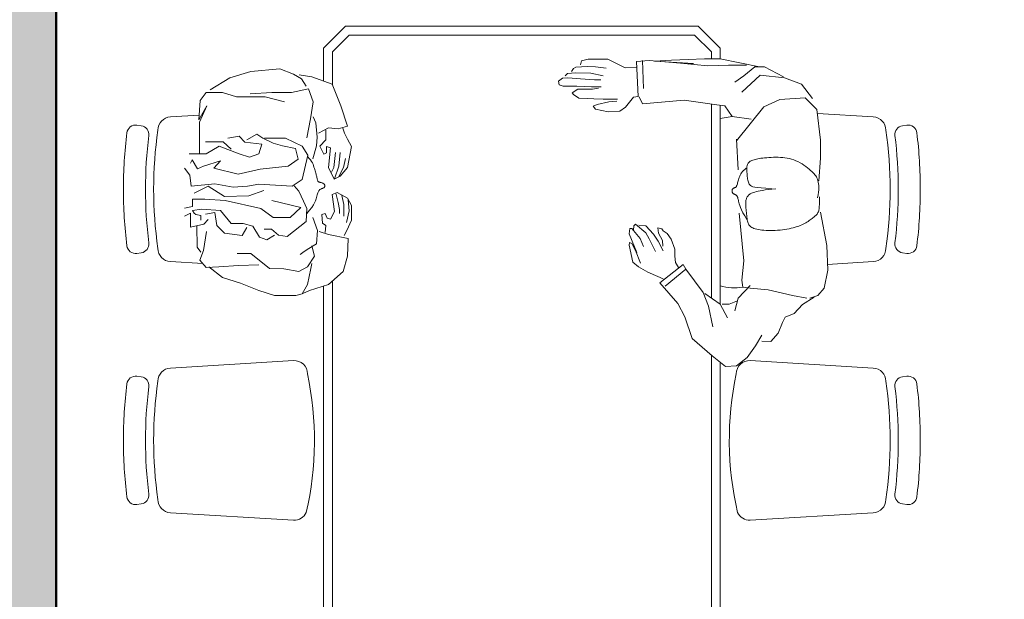
# Model space of a CAD drawing. Units: inches. Extents: x 1734 to 4011, y 1071 to 1891.
# Tile 20 of 27: x 3311 to 3379, y 1683 to 1723. Entities that reach past the tile are written whole.
import ezdxf

# ---------------------------------------------------------------- set-up
doc = ezdxf.new("R2010")
doc.units = ezdxf.units.IN
for name, color, linetype, lineweight in [('A-ANNO-DIMS', 2, 'Continuous', 18), ('A-FURN', 8, 'Continuous', 18), ('A-WALL', 7, 'Continuous', 50), ('A-WALL-PATT', 8, 'Continuous', 13)]:
    doc.layers.add(name, color=color, linetype=linetype, lineweight=lineweight)
doc.styles.get("Standard").update_dxf_attribs({"font": 'arial.ttf'})
doc.dimstyles.new('ISO-25', dxfattribs={"dimtxt": 5, "dimasz": 2.5, "dimexe": 1.25, "dimexo": 0.625, "dimtad": 1, "dimdec": 1, "dimlunit": 3, "dimtxsty": 'Standard', "dimcen": 2.5, "dimclrt": 1, "dimadec": 0, "dimazin": 0, "dimtfac": 1, "dimtdec": 1, "dimtmove": 0, "dimatfit": 3, "dimfxl": 1, "dimarcsym": 0})

# ---------------------------------------------------------------- blocks, each defined once
blk = doc.blocks.new('A$C421907B3')
for p, q in [((0.3928, 1.2157), (0.4173, 1.234)), ((0.4173, 1.234), (0.4418, 1.2361)), ((0.4418, 1.2361), (0.4726, 1.2115)), ((0.3742, 1.1891), (0.3928, 1.2157)), ((0.4726, 1.2115), (0.5176, 1.1724)), ((0.36, 1.1646), (0.3742, 1.1891)), ((0.3229, 1.1605), (0.3394, 1.1788)), ((0.3394, 1.1788), (0.36, 1.1787)), ((0.5176, 1.1724), (0.5341, 1.1234)), ((0.3126, 1.1359), (0.3229, 1.1605)), ((0.4808, 1.0989), (0.4706, 1.1459)), ((0.2861, 1.1152), (0.3066, 1.1235)), ((0.3066, 1.1235), (0.3126, 1.1359)), ((0.4378, 1.1255), (0.454, 1.0947)), ((0.5341, 1.1234), (0.5503, 1.0926)), ((0.2676, 1.0948), (0.2861, 1.1152)), ((0.4132, 1.0806), (0.4212, 1.1093)), ((0.493, 1.0681), (0.4808, 1.0989)), ((0.2328, 1.0745), (0.2183, 1.0579)), ((0.2511, 1.0807), (0.2328, 1.0745)), ((0.241, 1.0786), (0.2676, 1.0948)), ((0.2573, 1.0807), (0.2901, 1.0744)), ((0.2901, 1.0744), (0.3454, 1.062)), ((0.3864, 1.0516), (0.4132, 1.0806)), ((0.4335, 1.0947), (0.4152, 1.0865)), ((0.45, 1.0947), (0.4335, 1.0947)), ((0.454, 1.0947), (0.489, 1.0702)), ((0.5503, 1.0926), (0.5914, 1.0456)), ((1.4171, 1.0745), (1.4031, 1.0709)), ((1.4656, 1.0745), (1.4171, 1.0745)), ((1.5014, 1.0634), (1.4656, 1.0745)), ((0.2183, 1.0579), (0.2102, 1.0171)), ((0.3454, 1.062), (0.3864, 1.0578)), ((0.3864, 1.0578), (0.4029, 1.0557)), ((0.4029, 1.0557), (0.4049, 1.0395)), ((0.5322, 1.015), (0.493, 1.0681)), ((0.5791, 1.0535), (0.532, 1.0149)), ((1.3433, 1.0498), (1.3858, 1.0635)), ((1.3858, 1.0635), (1.4011, 1.0699)), ((1.4031, 1.0709), (1.3905, 1.0498)), ((1.5426, 1.0469), (1.5014, 1.0634)), ((0.4049, 1.0395), (0.4006, 0.9963)), ((0.538, 1.0045), (0.5914, 1.0456)), ((0.5958, 1.0315), (0.5832, 1.0366)), ((0.618, 1.0218), (0.5958, 1.0315)), ((1.3094, 1.0205), (1.3433, 1.0498)), ((1.3905, 1.0498), (1.3831, 1.0131)), ((1.5838, 1.034), (1.5426, 1.0469)), ((1.615, 1.0092), (1.5838, 1.034)), ((0.2102, 1.0171), (0.2122, 0.9615)), ((0.532, 1.0149), (0.538, 1.0045)), ((0.5491, 1.0108), (0.5557, 0.9996)), ((0.6395, 1.0092), (0.618, 1.0218)), ((0.6521, 0.9988), (0.6395, 1.0092)), ((1.3001, 0.9856), (1.3094, 1.0205)), ((1.3751, 0.9856), (1.3904, 1.0094)), ((1.3831, 1.0131), (1.3811, 1.0021)), ((1.3904, 1.0094), (1.4104, 1.0204)), ((1.4104, 1.0204), (1.4443, 1.0139)), ((1.4443, 1.0139), (1.4768, 1.013)), ((1.4768, 1.013), (1.5193, 0.979)), ((1.5014, 1.0047), (1.5472, 1.0065)), ((1.5472, 1.0065), (1.5918, 1.0092)), ((1.5918, 1.0092), (1.621, 1.011)), ((1.621, 1.011), (1.6349, 0.9945)), ((0.4006, 0.9963), (0.4108, 0.8878)), ((0.5557, 0.9996), (0.5572, 0.9855)), ((0.5572, 0.9855), (0.5572, 0.9693)), ((0.635, 1.001), (0.6461, 0.9722)), ((0.6609, 0.9603), (0.6521, 0.9988)), ((1.2987, 0.9453), (1.3001, 0.9856)), ((1.3811, 0.9617), (1.3751, 0.9856)), ((1.6349, 0.9945), (1.627, 0.9725)), ((0.2122, 0.9615), (0.2264, 0.8858)), ((0.5572, 0.9693), (0.5653, 0.947)), ((0.5832, 0.9729), (0.595, 0.9515)), ((0.5854, 0.9499), (0.5846, 0.9626)), ((0.6009, 0.9744), (0.615, 0.9462)), ((0.6283, 0.9633), (0.6357, 0.9455)), ((0.6609, 0.9344), (0.6432, 0.9774)), ((0.6461, 0.9722), (0.655, 0.9566)), ((1.3705, 0.9571), (1.3877, 0.9681)), ((1.3877, 0.9681), (1.3984, 0.9745)), ((1.3984, 0.9745), (1.4077, 0.9819)), ((1.5193, 0.979), (1.5505, 0.979)), ((1.627, 0.9725), (1.6196, 0.9294)), ((1.6409, 0.9652), (1.6329, 0.9762)), ((1.6421, 0.9163), (1.6409, 0.9652)), ((0.5653, 0.947), (0.5742, 0.9337)), ((0.5942, 0.933), (0.5854, 0.9499)), ((0.595, 0.9515), (0.6053, 0.9352)), ((0.615, 0.9462), (0.6232, 0.9322)), ((0.6357, 0.9455), (0.655, 0.9225)), ((0.655, 0.9566), (0.6602, 0.9544)), ((0.6602, 0.9544), (0.6609, 0.9603)), ((1.3432, 0.9361), (1.2987, 0.9453)), ((1.3013, 0.9269), (1.3073, 0.9388)), ((1.3678, 0.9269), (1.3705, 0.9571)), ((1.3937, 0.9067), (1.4369, 0.9406)), ((1.4369, 0.9406), (1.4568, 0.9378)), ((1.4655, 0.9378), (1.4827, 0.9479)), ((1.4827, 0.9479), (1.4994, 0.9423)), ((1.4994, 0.9423), (1.5146, 0.9176)), ((1.5286, 0.9203), (1.5392, 0.9386)), ((1.5392, 0.9386), (1.5791, 0.9331)), ((0.2723, 0.9155), (0.2759, 0.9169)), ((0.2759, 0.9169), (0.2797, 0.9183)), ((0.2797, 0.9183), (0.2839, 0.9196)), ((0.2839, 0.9196), (0.2883, 0.9208)), ((0.2883, 0.9208), (0.2929, 0.922)), ((0.2929, 0.922), (0.2977, 0.923)), ((0.2977, 0.923), (0.3027, 0.924)), ((0.3027, 0.924), (0.3078, 0.9248)), ((0.3078, 0.9248), (0.3131, 0.9255)), ((0.3131, 0.9255), (0.3184, 0.9261)), ((0.3184, 0.9261), (0.3238, 0.9266)), ((0.3238, 0.9266), (0.3293, 0.927)), ((0.3293, 0.927), (0.3347, 0.9272)), ((0.3347, 0.9272), (0.34, 0.9272)), ((0.34, 0.9272), (0.3452, 0.9272)), ((0.3452, 0.9272), (0.3502, 0.927)), ((0.3502, 0.927), (0.355, 0.9267)), ((0.355, 0.9267), (0.3595, 0.9262)), ((0.3595, 0.9262), (0.3638, 0.9257)), ((0.3638, 0.9257), (0.3677, 0.925)), ((0.3677, 0.925), (0.3713, 0.9242)), ((0.3713, 0.9242), (0.3746, 0.9233)), ((0.3746, 0.9233), (0.3776, 0.9223)), ((0.3776, 0.9223), (0.3803, 0.9212)), ((0.3803, 0.9212), (0.3826, 0.92)), ((0.3826, 0.92), (0.3847, 0.9187)), ((0.3847, 0.9187), (0.3864, 0.9173)), ((0.3864, 0.9173), (0.3878, 0.9158)), ((0.5742, 0.9337), (0.5832, 0.9278)), ((0.5832, 0.9278), (0.5869, 0.9233)), ((0.5869, 0.9233), (0.5957, 0.9211)), ((0.5957, 0.9211), (0.5942, 0.933)), ((0.6053, 0.9352), (0.6232, 0.9166)), ((0.6232, 0.9322), (0.6461, 0.9129)), ((0.6232, 0.9166), (0.6387, 0.9151)), ((0.6461, 0.9129), (0.6498, 0.9166)), ((0.6498, 0.9166), (0.6506, 0.9263)), ((0.655, 0.9225), (0.6594, 0.9225)), ((0.6594, 0.9225), (0.6609, 0.9344)), ((1.2907, 0.904), (1.3013, 0.9269)), ((1.3645, 0.9296), (1.3432, 0.9361)), ((1.3505, 0.9315), (1.3492, 0.9159)), ((1.3784, 0.8975), (1.3678, 0.9269)), ((1.4568, 0.9378), (1.4721, 0.924)), ((1.4721, 0.924), (1.4887, 0.924)), ((1.5146, 0.9176), (1.5365, 0.9111)), ((1.5791, 0.9331), (1.5963, 0.9157)), ((1.6256, 0.9129), (1.6561, 0.9193)), ((1.6561, 0.9193), (1.6561, 0.8881)), ((0.237, 0.8927), (0.2385, 0.8941)), ((0.2385, 0.8941), (0.2401, 0.8956)), ((0.2401, 0.8956), (0.2419, 0.897)), ((0.2419, 0.897), (0.2437, 0.8985)), ((0.2437, 0.8985), (0.2457, 0.9)), ((0.2457, 0.9), (0.2478, 0.9016)), ((0.2478, 0.9016), (0.25, 0.9031)), ((0.25, 0.9031), (0.2524, 0.9047)), ((0.2524, 0.9047), (0.2548, 0.9063)), ((0.2548, 0.9063), (0.2573, 0.9078)), ((0.2573, 0.9078), (0.26, 0.9094)), ((0.26, 0.9094), (0.2628, 0.911)), ((0.2628, 0.911), (0.2657, 0.9125)), ((0.2657, 0.9125), (0.2689, 0.914)), ((0.2689, 0.914), (0.2723, 0.9155)), ((0.3878, 0.9158), (0.389, 0.9142)), ((0.389, 0.9142), (0.39, 0.9123)), ((0.39, 0.9123), (0.3908, 0.9104)), ((0.3908, 0.9104), (0.3915, 0.9081)), ((0.3915, 0.9081), (0.3921, 0.9057)), ((0.3921, 0.9057), (0.3926, 0.903)), ((0.3926, 0.903), (0.3931, 0.8999)), ((0.3931, 0.8999), (0.3935, 0.8967)), ((0.3935, 0.8967), (0.394, 0.8933)), ((0.3936, 0.9023), (0.3986, 0.894)), ((0.3986, 0.894), (0.4026, 0.8867)), ((1.2906, 0.87), (1.2907, 0.904)), ((1.2965, 0.8821), (1.3022, 0.9091)), ((1.3079, 0.8681), (1.3079, 0.8945)), ((1.3385, 0.9012), (1.3292, 0.8838)), ((1.3458, 0.8994), (1.3385, 0.9012)), ((1.3505, 0.8883), (1.3458, 0.8994)), ((1.3492, 0.9159), (1.3565, 0.9104)), ((1.3565, 0.9104), (1.3584, 0.8911)), ((1.3923, 0.8773), (1.3937, 0.9067)), ((1.4056, 0.8745), (1.4302, 0.8974)), ((1.4302, 0.8974), (1.4687, 0.8974)), ((1.4687, 0.8974), (1.4966, 0.8772)), ((1.5365, 0.9111), (1.5638, 0.9111)), ((1.5638, 0.9111), (1.5883, 0.8817)), ((1.5963, 0.9157), (1.601, 0.8863)), ((1.6163, 0.9019), (1.6256, 0.9129)), ((1.6329, 0.8927), (1.6329, 0.9037)), ((1.6561, 0.8881), (1.6701, 0.8945)), ((0.2291, 0.8687), (0.2292, 0.8722)), ((0.2292, 0.8722), (0.2294, 0.8753)), ((0.2294, 0.8753), (0.2297, 0.8781)), ((0.2297, 0.8781), (0.2301, 0.8806)), ((0.2301, 0.8806), (0.2306, 0.8828)), ((0.2306, 0.8828), (0.2313, 0.8848)), ((0.2313, 0.8848), (0.2322, 0.8866)), ((0.2322, 0.8866), (0.2332, 0.8883)), ((0.2332, 0.8883), (0.2343, 0.8898)), ((0.2343, 0.8898), (0.2356, 0.8913)), ((0.2356, 0.8913), (0.237, 0.8927)), ((0.394, 0.8933), (0.3944, 0.8898)), ((0.3944, 0.8898), (0.3947, 0.8863)), ((0.3947, 0.8863), (0.3951, 0.8829)), ((0.3951, 0.8829), (0.3954, 0.8796)), ((0.3954, 0.8796), (0.3957, 0.8765)), ((0.3957, 0.8765), (0.3959, 0.8736)), ((0.3959, 0.8736), (0.3961, 0.871)), ((0.4026, 0.8867), (0.4057, 0.8804)), ((0.4057, 0.8804), (0.4081, 0.8751)), ((0.4081, 0.8751), (0.4098, 0.8705)), ((1.2985, 0.8577), (1.2965, 0.8821)), ((1.3183, 0.8795), (1.3183, 0.8888)), ((1.3209, 0.8634), (1.3183, 0.8795)), ((1.3292, 0.8838), (1.3351, 0.8452)), ((1.3584, 0.8911), (1.3505, 0.8883)), ((1.3774, 0.869), (1.3812, 0.8747)), ((1.3812, 0.8747), (1.3861, 0.8811)), ((1.3861, 0.8811), (1.3923, 0.8883)), ((1.3996, 0.8608), (1.3923, 0.8773)), ((1.472, 0.8589), (1.4056, 0.8745)), ((1.4966, 0.8772), (1.5777, 0.8588)), ((1.5883, 0.8817), (1.6315, 0.8789)), ((1.601, 0.8863), (1.6222, 0.8899)), ((1.6315, 0.8789), (1.6515, 0.8817)), ((1.6442, 0.8908), (1.6329, 0.8927)), ((1.6481, 0.8881), (1.6442, 0.8908)), ((1.6515, 0.8817), (1.6481, 0.8881)), ((1.6514, 0.8725), (1.6701, 0.8761)), ((1.6514, 0.856), (1.6514, 0.8725)), ((0.2291, 0.8649), (0.2291, 0.8687)), ((0.2291, 0.8607), (0.2291, 0.8649)), ((0.2291, 0.856), (0.2291, 0.8607)), ((0.2291, 0.8509), (0.2291, 0.856)), ((0.2316, 0.8463), (0.2331, 0.8527)), ((0.3918, 0.8495), (0.3909, 0.8482)), ((0.3927, 0.8508), (0.3918, 0.8495)), ((0.3934, 0.8523), (0.3927, 0.8508)), ((0.3941, 0.8538), (0.3934, 0.8523)), ((0.3947, 0.8553), (0.3941, 0.8538)), ((0.3952, 0.857), (0.3947, 0.8553)), ((0.3956, 0.8587), (0.3952, 0.857)), ((0.3959, 0.8604), (0.3956, 0.8587)), ((0.3961, 0.8623), (0.3959, 0.8604)), ((0.3961, 0.871), (0.3962, 0.8685)), ((0.3962, 0.8642), (0.3961, 0.8623)), ((0.3962, 0.8685), (0.3962, 0.8663)), ((0.3962, 0.8663), (0.3962, 0.8642)), ((0.4098, 0.8705), (0.411, 0.8667)), ((0.411, 0.8667), (0.4118, 0.8634)), ((0.4118, 0.8634), (0.4124, 0.8607)), ((0.4124, 0.8607), (0.4129, 0.8583)), ((0.4129, 0.8583), (0.4134, 0.8564)), ((0.4134, 0.8564), (0.4138, 0.8547)), ((0.4138, 0.8547), (0.4141, 0.8533)), ((0.4141, 0.8533), (0.4145, 0.8522)), ((0.4145, 0.8522), (0.4148, 0.8512)), ((0.4148, 0.8512), (0.4152, 0.8504)), ((0.4152, 0.8504), (0.4156, 0.8497)), ((0.4156, 0.8497), (0.416, 0.849)), ((1.2999, 0.8535), (1.2906, 0.87)), ((1.3232, 0.8407), (1.2999, 0.8535)), ((1.3126, 0.8473), (1.3079, 0.8681)), ((1.3261, 0.8427), (1.3209, 0.8634)), ((1.3694, 0.849), (1.3702, 0.852)), ((1.3702, 0.852), (1.3712, 0.8555)), ((1.3712, 0.8555), (1.3726, 0.8595)), ((1.3726, 0.8595), (1.3746, 0.864)), ((1.3746, 0.864), (1.3774, 0.869)), ((1.4102, 0.8378), (1.3996, 0.8608)), ((1.5239, 0.8487), (1.579, 0.8496)), ((1.5777, 0.8588), (1.6235, 0.856)), ((1.579, 0.8496), (1.6162, 0.8266)), ((1.6235, 0.856), (1.6514, 0.856)), ((0.2301, 0.8299), (0.2302, 0.8349)), ((0.2304, 0.8252), (0.2301, 0.8299)), ((0.2302, 0.8349), (0.2307, 0.8404)), ((0.2307, 0.8404), (0.2316, 0.8463)), ((0.3369, 0.8333), (0.328, 0.8326)), ((0.3448, 0.8341), (0.3369, 0.8333)), ((0.3375, 0.8319), (0.3508, 0.8313)), ((0.3518, 0.835), (0.3448, 0.8341)), ((0.3508, 0.8313), (0.3614, 0.8306)), ((0.3579, 0.8359), (0.3518, 0.835)), ((0.3632, 0.8369), (0.3579, 0.8359)), ((0.3614, 0.8306), (0.3695, 0.8298)), ((0.3678, 0.8379), (0.3632, 0.8369)), ((0.3718, 0.8389), (0.3678, 0.8379)), ((0.3695, 0.8298), (0.3757, 0.8289)), ((0.3752, 0.8398), (0.3718, 0.8389)), ((0.3782, 0.8407), (0.3752, 0.8398)), ((0.3757, 0.8289), (0.3801, 0.8278)), ((0.3807, 0.8416), (0.3782, 0.8407)), ((0.3801, 0.8278), (0.3832, 0.8265)), ((0.3829, 0.8425), (0.3807, 0.8416)), ((0.3847, 0.8433), (0.3829, 0.8425)), ((0.3863, 0.8442), (0.3847, 0.8433)), ((0.3876, 0.8451), (0.3863, 0.8442)), ((0.3888, 0.846), (0.3876, 0.8451)), ((0.3899, 0.8471), (0.3888, 0.846)), ((0.3909, 0.8482), (0.3899, 0.8471)), ((0.416, 0.849), (0.4165, 0.8484)), ((0.4165, 0.8484), (0.417, 0.8478)), ((0.4173, 0.827), (0.4168, 0.826)), ((0.417, 0.8478), (0.4176, 0.8473)), ((0.4178, 0.8277), (0.4173, 0.827)), ((0.4176, 0.8473), (0.4182, 0.8468)), ((0.4183, 0.8283), (0.4178, 0.8277)), ((0.4182, 0.8468), (0.4188, 0.8463)), ((0.4188, 0.8288), (0.4183, 0.8283)), ((0.4188, 0.8463), (0.4195, 0.8459)), ((0.4194, 0.8291), (0.4188, 0.8288)), ((0.42, 0.8294), (0.4194, 0.8291)), ((0.4195, 0.8459), (0.4202, 0.8455)), ((0.4207, 0.8297), (0.42, 0.8294)), ((0.4202, 0.8455), (0.4209, 0.8451)), ((0.4215, 0.83), (0.4207, 0.8297)), ((0.4209, 0.8451), (0.4217, 0.8448)), ((0.4223, 0.8303), (0.4215, 0.83)), ((0.4217, 0.8448), (0.4225, 0.8444)), ((0.4231, 0.8307), (0.4223, 0.8303)), ((0.4225, 0.8444), (0.4233, 0.8439)), ((0.424, 0.8311), (0.4231, 0.8307)), ((0.4233, 0.8439), (0.424, 0.8435)), ((0.424, 0.8435), (0.4247, 0.8429)), ((0.4248, 0.8316), (0.424, 0.8311)), ((0.4247, 0.8429), (0.4253, 0.8423)), ((0.4255, 0.8322), (0.4248, 0.8316)), ((0.4253, 0.8423), (0.4259, 0.8415)), ((0.4261, 0.8329), (0.4255, 0.8322)), ((0.4259, 0.8415), (0.4264, 0.8407)), ((0.4267, 0.8337), (0.4261, 0.8329)), ((0.4264, 0.8407), (0.4268, 0.8397)), ((0.427, 0.8346), (0.4267, 0.8337)), ((0.4268, 0.8397), (0.4271, 0.8387)), ((0.4272, 0.8356), (0.427, 0.8346)), ((0.4271, 0.8387), (0.4273, 0.8377)), ((0.4273, 0.8366), (0.4272, 0.8356)), ((0.4273, 0.8377), (0.4273, 0.8366)), ((1.3351, 0.8452), (1.3232, 0.8407)), ((1.3512, 0.826), (1.3514, 0.8269)), ((1.3514, 0.8269), (1.3518, 0.8277)), ((1.3518, 0.8277), (1.3524, 0.8285)), ((1.3524, 0.8285), (1.353, 0.8292)), ((1.353, 0.8292), (1.3538, 0.8299)), ((1.3538, 0.8299), (1.3547, 0.8305)), ((1.3547, 0.8305), (1.3557, 0.8311)), ((1.3557, 0.8311), (1.3568, 0.8316)), ((1.3568, 0.8316), (1.3579, 0.832)), ((1.3579, 0.832), (1.3591, 0.8325)), ((1.3591, 0.8325), (1.3602, 0.833)), ((1.3602, 0.833), (1.3613, 0.8335)), ((1.3613, 0.8335), (1.3624, 0.8342)), ((1.3624, 0.8342), (1.3634, 0.835)), ((1.3634, 0.835), (1.3643, 0.8359)), ((1.3643, 0.8359), (1.3651, 0.837)), ((1.3651, 0.837), (1.3659, 0.8384)), ((1.3659, 0.8384), (1.3666, 0.8399)), ((1.3666, 0.8399), (1.3673, 0.8417)), ((1.3673, 0.8417), (1.368, 0.8438)), ((1.368, 0.8438), (1.3687, 0.8462)), ((1.3687, 0.8462), (1.3694, 0.849)), ((1.4029, 0.8112), (1.4255, 0.8268)), ((1.4208, 0.8259), (1.4102, 0.8378)), ((1.4255, 0.8268), (1.5012, 0.8222)), ((1.49, 0.8359), (1.5239, 0.8487)), ((1.5272, 0.8267), (1.5591, 0.8285)), ((1.5591, 0.8285), (1.6009, 0.8212)), ((1.6162, 0.8266), (1.6481, 0.8422)), ((0.2306, 0.814), (0.2263, 0.7628)), ((0.2309, 0.821), (0.2304, 0.8252)), ((0.2316, 0.8172), (0.2309, 0.821)), ((0.2325, 0.8138), (0.2316, 0.8172)), ((0.2335, 0.8107), (0.2325, 0.8138)), ((0.2346, 0.8079), (0.2335, 0.8107)), ((0.2359, 0.8053), (0.2346, 0.8079)), ((0.2374, 0.8029), (0.2359, 0.8053)), ((0.3832, 0.8265), (0.3854, 0.8251)), ((0.3854, 0.8251), (0.3869, 0.8235)), ((0.3869, 0.8235), (0.3882, 0.8218)), ((0.3882, 0.8218), (0.3892, 0.8198)), ((0.3892, 0.8198), (0.3901, 0.8176)), ((0.3901, 0.8176), (0.3908, 0.8153)), ((0.3908, 0.8153), (0.3914, 0.8128)), ((0.3914, 0.8128), (0.3919, 0.8101)), ((0.3919, 0.8101), (0.3923, 0.8073)), ((0.3923, 0.8073), (0.3926, 0.8043)), ((0.4108, 0.8066), (0.4098, 0.804)), ((0.4117, 0.8093), (0.4108, 0.8066)), ((0.4126, 0.8119), (0.4117, 0.8093)), ((0.4133, 0.8145), (0.4126, 0.8119)), ((0.414, 0.8169), (0.4133, 0.8145)), ((0.4147, 0.8192), (0.414, 0.8169)), ((0.4152, 0.8213), (0.4147, 0.8192)), ((0.4158, 0.8231), (0.4152, 0.8213)), ((0.4163, 0.8247), (0.4158, 0.8231)), ((0.4168, 0.826), (0.4163, 0.8247)), ((1.3089, 0.784), (1.3203, 0.8058)), ((1.3165, 0.804), (1.3305, 0.8104)), ((1.3193, 0.7809), (1.3297, 0.8099)), ((1.3305, 0.8104), (1.3431, 0.7838)), ((1.3512, 0.8251), (1.3512, 0.826)), ((1.3514, 0.8243), (1.3512, 0.8251)), ((1.3518, 0.8234), (1.3514, 0.8243)), ((1.3524, 0.8226), (1.3518, 0.8234)), ((1.3531, 0.8218), (1.3524, 0.8226)), ((1.354, 0.8211), (1.3531, 0.8218)), ((1.355, 0.8204), (1.354, 0.8211)), ((1.3561, 0.8198), (1.355, 0.8204)), ((1.3572, 0.8192), (1.3561, 0.8198)), ((1.3584, 0.8188), (1.3572, 0.8192)), ((1.3595, 0.8184), (1.3584, 0.8188)), ((1.3607, 0.8181), (1.3595, 0.8184)), ((1.3618, 0.8179), (1.3607, 0.8181)), ((1.3629, 0.8176), (1.3618, 0.8179)), ((1.3639, 0.8173), (1.3629, 0.8176)), ((1.3648, 0.8169), (1.3639, 0.8173)), ((1.3656, 0.8165), (1.3648, 0.8169)), ((1.3664, 0.8159), (1.3656, 0.8165)), ((1.367, 0.8151), (1.3664, 0.8159)), ((1.3675, 0.8141), (1.367, 0.8151)), ((1.3679, 0.813), (1.3675, 0.8141)), ((1.3683, 0.8118), (1.3679, 0.813)), ((1.3686, 0.8104), (1.3683, 0.8118)), ((1.369, 0.8088), (1.3686, 0.8104)), ((1.3694, 0.8071), (1.369, 0.8088)), ((1.3698, 0.8053), (1.3694, 0.8071)), ((1.3703, 0.8033), (1.3698, 0.8053)), ((1.3902, 0.7562), (1.4029, 0.8112)), ((1.5012, 0.8222), (1.5272, 0.8267)), ((1.6009, 0.8212), (1.6547, 0.8266)), ((1.6547, 0.8266), (1.6574, 0.8018)), ((0.2391, 0.8006), (0.2374, 0.8029)), ((0.241, 0.7983), (0.2391, 0.8006)), ((0.2433, 0.7958), (0.241, 0.7983)), ((0.246, 0.7933), (0.2433, 0.7958)), ((0.249, 0.7905), (0.246, 0.7933)), ((0.2523, 0.7876), (0.249, 0.7905)), ((0.256, 0.7846), (0.2523, 0.7876)), ((0.2599, 0.7816), (0.256, 0.7846)), ((0.3926, 0.8043), (0.393, 0.8012)), ((0.393, 0.8012), (0.3933, 0.7979)), ((0.3934, 0.7825), (0.393, 0.7799)), ((0.3933, 0.7979), (0.3936, 0.7947)), ((0.3937, 0.7853), (0.3934, 0.7825)), ((0.3936, 0.7947), (0.3937, 0.7915)), ((0.3937, 0.7915), (0.3938, 0.7883)), ((0.3938, 0.7883), (0.3937, 0.7853)), ((0.3986, 0.7884), (0.3953, 0.7859)), ((0.4014, 0.7909), (0.3986, 0.7884)), ((0.4037, 0.7935), (0.4014, 0.7909)), ((0.4057, 0.796), (0.4037, 0.7935)), ((0.4073, 0.7987), (0.4057, 0.796)), ((0.4087, 0.8013), (0.4073, 0.7987)), ((0.4098, 0.804), (0.4087, 0.8013)), ((0.413, 0.7893), (0.417, 0.7199)), ((1.2905, 0.7361), (1.2999, 0.7838)), ((1.2999, 0.7838), (1.3165, 0.804)), ((1.3047, 0.7638), (1.3089, 0.784)), ((1.3275, 0.7498), (1.3307, 0.784)), ((1.3307, 0.784), (1.3359, 0.7949)), ((1.3431, 0.7838), (1.3384, 0.7397)), ((1.3708, 0.8013), (1.3703, 0.8033)), ((1.3714, 0.799), (1.3708, 0.8013)), ((1.3721, 0.7967), (1.3714, 0.799)), ((1.3728, 0.7942), (1.3721, 0.7967)), ((1.3736, 0.7916), (1.3728, 0.7942)), ((1.3743, 0.7889), (1.3736, 0.7916)), ((1.3751, 0.786), (1.3743, 0.7889)), ((1.376, 0.783), (1.3751, 0.786)), ((1.3769, 0.7799), (1.376, 0.783)), ((1.4348, 0.7809), (1.4979, 0.7882)), ((1.4979, 0.7882), (1.5484, 0.7992)), ((1.5484, 0.7992), (1.6035, 0.7854)), ((1.6035, 0.7854), (1.5882, 0.7689)), ((1.6268, 0.7808), (1.6407, 0.7872)), ((1.6407, 0.7872), (1.6527, 0.767)), ((1.6574, 0.8018), (1.67, 0.7853)), ((0.2263, 0.7628), (0.2263, 0.7217)), ((0.264, 0.7786), (0.2599, 0.7816)), ((0.2684, 0.7758), (0.264, 0.7786)), ((0.2729, 0.7731), (0.2684, 0.7758)), ((0.2776, 0.7707), (0.2729, 0.7731)), ((0.2823, 0.7686), (0.2776, 0.7707)), ((0.2871, 0.7668), (0.2823, 0.7686)), ((0.292, 0.7652), (0.2871, 0.7668)), ((0.297, 0.764), (0.292, 0.7652)), ((0.302, 0.7629), (0.297, 0.764)), ((0.3071, 0.7621), (0.302, 0.7629)), ((0.3123, 0.7616), (0.3071, 0.7621)), ((0.3176, 0.7612), (0.3123, 0.7616)), ((0.3229, 0.7609), (0.3176, 0.7612)), ((0.3282, 0.7609), (0.3229, 0.7609)), ((0.3335, 0.7609), (0.3282, 0.7609)), ((0.3387, 0.7611), (0.3335, 0.7609)), ((0.3438, 0.7614), (0.3387, 0.7611)), ((0.3486, 0.7618), (0.3438, 0.7614)), ((0.3533, 0.7622), (0.3486, 0.7618)), ((0.3576, 0.7627), (0.3533, 0.7622)), ((0.3617, 0.7632), (0.3576, 0.7627)), ((0.3654, 0.7637), (0.3617, 0.7632)), ((0.3688, 0.7643), (0.3654, 0.7637)), ((0.3719, 0.7649), (0.3688, 0.7643)), ((0.3748, 0.7656), (0.3719, 0.7649)), ((0.3774, 0.7663), (0.3748, 0.7656)), ((0.3799, 0.7671), (0.3774, 0.7663)), ((0.3821, 0.768), (0.3799, 0.7671)), ((0.3841, 0.7689), (0.3821, 0.768)), ((0.386, 0.7699), (0.3841, 0.7689)), ((0.3876, 0.7711), (0.386, 0.7699)), ((0.3891, 0.7724), (0.3876, 0.7711)), ((0.3904, 0.7739), (0.3891, 0.7724)), ((0.3914, 0.7756), (0.3904, 0.7739)), ((0.3923, 0.7776), (0.3914, 0.7756)), ((0.393, 0.7799), (0.3923, 0.7776)), ((1.3166, 0.7498), (1.3193, 0.7809)), ((1.3703, 0.7351), (1.3783, 0.7645)), ((1.378, 0.7767), (1.3769, 0.7799)), ((1.3795, 0.7735), (1.378, 0.7767)), ((1.3813, 0.7701), (1.3795, 0.7735)), ((1.3837, 0.7667), (1.3813, 0.7701)), ((1.3866, 0.7633), (1.3837, 0.7667)), ((1.3902, 0.7599), (1.3866, 0.7633)), ((1.4122, 0.7654), (1.4348, 0.7809)), ((1.4181, 0.7406), (1.4122, 0.7654)), ((1.5012, 0.7534), (1.5224, 0.7607)), ((1.5224, 0.7607), (1.5457, 0.7533)), ((1.5882, 0.7689), (1.6268, 0.7808)), ((1.6527, 0.767), (1.656, 0.7743)), ((1.3384, 0.7397), (1.3477, 0.7361)), ((1.3477, 0.7507), (1.3537, 0.7535)), ((1.3477, 0.7361), (1.3477, 0.7507)), ((1.3537, 0.7535), (1.363, 0.736)), ((1.4028, 0.736), (1.3902, 0.7562)), ((1.4473, 0.7351), (1.4181, 0.7406)), ((1.4945, 0.7313), (1.5012, 0.7534)), ((1.5457, 0.7533), (1.5915, 0.7358)), ((1.5822, 0.7258), (1.5636, 0.7423)), ((1.5915, 0.7358), (1.6208, 0.7532)), ((1.6208, 0.7532), (1.6593, 0.7532)), ((1.6361, 0.7532), (1.636, 0.6808)), ((0.2263, 0.7217), (0.2345, 0.6523)), ((0.3554, 0.646), (0.417, 0.7237)), ((1.2998, 0.7196), (1.2905, 0.7361)), ((1.3071, 0.7058), (1.2998, 0.7196)), ((1.363, 0.736), (1.349, 0.7214)), ((1.349, 0.7214), (1.349, 0.6984)), ((1.3689, 0.7149), (1.3703, 0.7351)), ((1.3842, 0.6736), (1.3922, 0.7167)), ((1.4407, 0.7176), (1.4028, 0.736)), ((1.4885, 0.7176), (1.4407, 0.7176)), ((1.4686, 0.7286), (1.4473, 0.7351)), ((1.4918, 0.7176), (1.4686, 0.7286)), ((1.5058, 0.7084), (1.4918, 0.7176)), ((1.5331, 0.7267), (1.4945, 0.7313)), ((1.5284, 0.7212), (1.5058, 0.7084)), ((1.5457, 0.7129), (1.5331, 0.7267)), ((1.5716, 0.7175), (1.5457, 0.7129)), ((1.6221, 0.7257), (1.5822, 0.7258)), ((1.2998, 0.6902), (1.3211, 0.6966)), ((1.3104, 0.6948), (1.3071, 0.7058)), ((1.3211, 0.6966), (1.343, 0.6939)), ((1.343, 0.6939), (1.3656, 0.7058)), ((1.3716, 0.6828), (1.3689, 0.7149)), ((0.3842, 0.6746), (0.4272, 0.6684)), ((0.4272, 0.6684), (0.4542, 0.6729)), ((1.315, 0.6443), (1.2998, 0.6902)), ((1.3782, 0.6691), (1.3716, 0.6828)), ((1.3782, 0.6351), (1.3842, 0.6736)), ((1.636, 0.6808), (1.6194, 0.6441)), ((1.6194, 0.6441), (1.6373, 0.6762)), ((1.6373, 0.6762), (1.6346, 0.6321)), ((0.2345, 0.6523), (0.261, 0.6256)), ((0.4272, 0.6684), (0.4435, 0.6438)), ((0.6692, 0.647), (0.6821, 0.6561)), ((0.6821, 0.6561), (0.7085, 0.6576)), ((0.7085, 0.6576), (0.7372, 0.6515)), ((0.7372, 0.6515), (0.7425, 0.6447)), ((0.2448, 0.6277), (0.2693, 0.5949)), ((0.261, 0.6256), (0.3186, 0.6294)), ((0.3186, 0.6294), (0.3554, 0.646)), ((0.4435, 0.6438), (0.462, 0.6418)), ((0.462, 0.6418), (0.5358, 0.6313)), ((0.5358, 0.6313), (0.6302, 0.6396)), ((0.6302, 0.6396), (0.6381, 0.6233)), ((0.6511, 0.6244), (0.6692, 0.647)), ((0.6873, 0.6288), (0.7199, 0.6288)), ((0.707, 0.6349), (0.6889, 0.6334)), ((0.7335, 0.6409), (0.707, 0.6349)), ((0.7199, 0.6288), (0.741, 0.6281)), ((0.7425, 0.6447), (0.7335, 0.6409)), ((0.741, 0.6281), (0.7546, 0.6273)), ((0.7546, 0.6273), (0.775, 0.6265)), ((0.775, 0.6265), (0.787, 0.6183)), ((1.3349, 0.5948), (1.315, 0.6443)), ((1.3888, 0.6057), (1.3782, 0.6351)), ((1.4871, 0.624), (1.4426, 0.6351)), ((1.6346, 0.6321), (1.6207, 0.6138)), ((0.3636, 0.5741), (0.4047, 0.6131)), ((0.6281, 0.6047), (0.6301, 0.5411)), ((0.6405, 0.6229), (0.6511, 0.6244)), ((0.6405, 0.6229), (0.6444, 0.5432)), ((0.744, 0.6062), (0.7304, 0.6039)), ((0.7621, 0.6062), (0.744, 0.6062)), ((0.7772, 0.6062), (0.7621, 0.6062)), ((0.7901, 0.6144), (0.7772, 0.6062)), ((0.787, 0.6183), (0.7901, 0.6144)), ((1.4273, 0.614), (1.3888, 0.6057)), ((1.4718, 0.6139), (1.4273, 0.614)), ((1.521, 0.6166), (1.4718, 0.6139)), ((1.5516, 0.624), (1.4871, 0.624)), ((1.5835, 0.6138), (1.5516, 0.624)), ((1.6114, 0.6074), (1.5668, 0.5808)), ((1.6207, 0.6138), (1.5835, 0.6138)), ((0.2693, 0.5949), (0.3083, 0.5804)), ((0.4004, 0.5761), (0.4209, 0.5906)), ((0.7243, 0.6009), (0.7462, 0.6009)), ((0.7395, 0.585), (0.7251, 0.585)), ((0.7712, 0.5828), (0.7395, 0.585)), ((0.7462, 0.6009), (0.7795, 0.5993)), ((0.7999, 0.5804), (0.7712, 0.5828)), ((0.7795, 0.5993), (0.8105, 0.5993)), ((0.8119, 0.5812), (0.7999, 0.5804)), ((0.8105, 0.5993), (0.8195, 0.5963)), ((0.8211, 0.588), (0.8119, 0.5812)), ((0.8195, 0.5963), (0.8211, 0.588)), ((1.3808, 0.5782), (1.3349, 0.5948)), ((1.404, 0.5828), (1.3934, 0.5993)), ((1.4226, 0.5718), (1.404, 0.5828)), ((0.3083, 0.5804), (0.3636, 0.5741)), ((0.3103, 0.5783), (0.3533, 0.5558)), ((0.3759, 0.5558), (0.4004, 0.5761)), ((0.7198, 0.576), (0.7477, 0.5699)), ((0.7477, 0.5699), (0.7825, 0.5691)), ((0.7817, 0.5563), (0.787, 0.5593)), ((0.7825, 0.5691), (0.8006, 0.5707)), ((0.787, 0.5593), (0.7916, 0.5661)), ((0.8006, 0.5707), (0.8059, 0.576)), ((1.41, 0.5736), (1.3808, 0.5782)), ((1.4532, 0.5598), (1.4226, 0.5718)), ((1.519, 0.5662), (1.4532, 0.5598)), ((1.5668, 0.5808), (1.519, 0.5662)), ((0.3533, 0.5558), (0.3759, 0.5558)), ((0.4543, 0.5377), (0.3646, 0.5558)), ((0.4354, 0.5516), (0.3944, 0.5516)), ((0.4825, 0.5536), (0.4354, 0.5516)), ((0.544, 0.5474), (0.4825, 0.5536)), ((0.6156, 0.5411), (0.544, 0.5474)), ((0.6444, 0.5432), (0.6156, 0.5411)), ((0.645, 0.5564), (0.6699, 0.5579)), ((0.6699, 0.5579), (0.6926, 0.5466)), ((0.6926, 0.5466), (0.7092, 0.5382)), ((0.7092, 0.5382), (0.7538, 0.5382)), ((0.713, 0.5586), (0.7372, 0.5555)), ((0.7372, 0.5555), (0.756, 0.5548)), ((0.7538, 0.5382), (0.7689, 0.5419)), ((0.756, 0.5548), (0.7817, 0.5563)), ((0.7689, 0.5419), (0.7711, 0.551))]:
    blk.add_line(p, q)
at = {"ltscale": 0.1}
for points in [[(0.4542, 1.2262), (0.4542, 2.2936), (0.5042, 2.3436), (0.5562, 2.3436)], [(1.2446, 2.3436), (1.3042, 2.3436), (1.3542, 2.2936), (1.3542, 1.0533)], [(0.4742, 1.2101), (0.4742, 2.2853), (0.5125, 2.3236), (0.5723, 2.3236)], [(1.245, 2.3234), (1.2959, 2.3236), (1.3342, 2.2853), (1.3342, 1.0419)], [(0.4542, 0.6426), (0.4542, 1.0946)], [(0.4742, 0.64), (0.4742, 1.0806)], [(1.3542, 0.5878), (1.3542, 0.5135), (1.3042, 0.4635), (0.5042, 0.4635), (0.4542, 0.5135), (0.4542, 0.5377)], [(1.3342, 0.5966), (1.3342, 0.5218), (1.2959, 0.4835), (0.5125, 0.4835), (0.4742, 0.5218), (0.4742, 0.5375)]]:
    blk.add_lwpolyline(points, dxfattribs=at)
for points in [[(0.0782, 1.5378, -0.399285), (0.1067, 1.5678), (0.3861, 1.5847, -0.305593), (0.4148, 1.5674, -0.109362), (0.4176, 1.2524, -0.429301), (0.3861, 1.2224), (0.1067, 1.2393, -0.399285), (0.0782, 1.2693, -0.071734)], [(1.7302, 1.5378, 0.399285), (1.7017, 1.5678), (1.4223, 1.5847, 0.305593), (1.3936, 1.5674, 0.109362), (1.3908, 1.2524, 0.429301), (1.4223, 1.2224), (1.7017, 1.2393, 0.399285), (1.7302, 1.2693, 0.071734)], [(0.05, 1.4036, 0.030867), (0.0575, 1.2816, -0.408428), (0.0405, 1.2593), (0.0306, 1.2579, -0.419966), (0.0079, 1.2752, -0.030916), (0, 1.4036, -0.030916), (0.0079, 1.5319, -0.419966), (0.0306, 1.5492), (0.0405, 1.5478, -0.408428), (0.0575, 1.5255, 0.030867)], [(1.7584, 1.4036, -0.030867), (1.7509, 1.2816, 0.408428), (1.7679, 1.2593), (1.7778, 1.2579, 0.419966), (1.8005, 1.2752, 0.030916), (1.8084, 1.4036, 0.030916), (1.8005, 1.5319, 0.419966), (1.7778, 1.5492), (1.7679, 1.5478, 0.408428), (1.7509, 1.5255, -0.030867)], [(0.05, 0.8335, -0.030867), (0.0575, 0.9554, 0.408428), (0.0405, 0.9777), (0.0306, 0.9791, 0.419966), (0.0079, 0.9618, 0.030916), (0, 0.8335, 0.030916), (0.0079, 0.7052, 0.419966), (0.0306, 0.6878), (0.0405, 0.6893, 0.408428), (0.0575, 0.7115, -0.030867)], [(1.7584, 0.8335, 0.030867), (1.7509, 0.9554, -0.408428), (1.7679, 0.9777), (1.7778, 0.9791, -0.419966), (1.8005, 0.9618, -0.030916), (1.8084, 0.8335, -0.030916), (1.8005, 0.7052, -0.419966), (1.7778, 0.6878), (1.7679, 0.6893, -0.408428), (1.7509, 0.7115, 0.030867)]]:
    blk.add_lwpolyline(points, format="xyb", close=True, dxfattribs=at)
for points in [[(0.2107, 1.004), (0.1067, 0.9977, 0.399285), (0.0782, 0.9677, 0.071734), (0.0782, 0.6992, 0.399285), (0.1067, 0.6693), (0.2334, 0.6616)], [(1.6285, 1.0021), (1.7017, 0.9977, -0.399285), (1.7302, 0.9677, -0.071734), (1.7302, 0.6992, -0.399285), (1.7017, 0.6693), (1.6367, 0.6653)]]:
    blk.add_lwpolyline(points, format="xyb", dxfattribs=at)
blk.add_lwpolyline([(0.5267, 0.5491), (0.5148, 0.5482), (0.6033, 0.5427), (0.6033, 0.5427), (0.5647, 0.5405), (0.5267, 0.5387), (0.4898, 0.5376), (0.4542, 0.5371)])
blk.add_arc((0.4222, 0.9527), 0.1048, 72.2191, 100.5893)
blk = doc.blocks.new('*D99')
at = {"layer": 'A-ANNO-DIMS', "color": 0, "lineweight": -2, "transparency": 16777216}
for p, q in [((3317.994, 1736.234), (3304.669, 1736.234)), ((3305.919, 1733.734), (3305.919, 1654.07)), ((3317.994, 1651.57), (3304.669, 1651.57)), ((3305.919, 1651.57), (3305.919, 1564.027))]:
    blk.add_line(p, q, dxfattribs=at)
at = {"layer": 'A-ANNO-DIMS', "color": 0, "transparency": 16777216}
for points in [[(3305.503, 1733.734), (3306.336, 1733.734), (3305.919, 1736.234)], [(3305.503, 1654.07), (3306.336, 1654.07), (3305.919, 1651.57)]]:
    blk.add_solid(points, dxfattribs=at)
at = {"layer": 'Defpoints', "color": 0, "transparency": 16777216}
for p in [(3318.619, 1736.234), (3305.919, 1651.57), (3318.619, 1651.57)]:
    blk.add_point(p, dxfattribs=at)
at = {"layer": 'A-ANNO-DIMS', "color": 1, "transparency": 16777216, "insert": (3302.709, 1606.548), "char_height": 5, "attachment_point": 5, "rotation": 90}
blk.add_mtext('DINING SET 7\'-0 1/2" TYP.', dxfattribs=at)

msp = doc.modelspace()

# ---------------------------------------------------------------- hatches: boundary and pattern name
at = {"layer": 'A-WALL-PATT'}
h = msp.add_hatch(color=256, dxfattribs=at)
h.dxf.hatch_style = 1
h.paths.add_polyline_path([(3475.994, 1831.819), (3115.994, 1831.819), (3115.994, 1745.819), (3130.994, 1745.819), (3130.994, 1750.819), (3124.994, 1750.819), (3124.994, 1822.819), (3214.994, 1822.819), (3214.994, 1780.819), (3219.994, 1780.819), (3219.994, 1822.819), (3308.994, 1822.819), (3308.994, 1750.819), (3254.994, 1750.819), (3254.994, 1745.819), (3308.994, 1745.819), (3308.994, 1604.819), (3313.994, 1604.819), (3313.994, 1745.819), (3366.994, 1745.819), (3366.994, 1750.819), (3313.994, 1750.819), (3313.994, 1822.819), (3401.994, 1822.819), (3401.994, 1750.819), (3396.994, 1750.819), (3396.994, 1745.819), (3411.994, 1745.819), (3411.994, 1750.819), (3406.994, 1750.819), (3406.994, 1822.819), (3466.994, 1822.819), (3466.994, 1750.819), (3441.994, 1750.819), (3441.994, 1745.819), (3466.994, 1745.819), (3466.994, 1517.819), (3452.494, 1517.819), (3452.494, 1512.819), (3466.994, 1512.819), (3466.994, 1458.819), (3446.494, 1458.819), (3446.494, 1453.819), (3466.994, 1453.819), (3466.994, 1237.819), (3372.994, 1237.819), (3372.994, 1228.819), (3466.994, 1228.819), (3466.994, 1120.819), (3309.994, 1120.819), (3309.994, 1184.819), (3310.994, 1184.819), (3310.994, 1189.819), (3303.994, 1189.819), (3303.994, 1120.819), (3291.994, 1120.819), (3291.994, 1111.819), (3475.994, 1111.819)])
h.paths.add_polyline_path([(3169.994, 1745.819), (3224.994, 1745.819), (3224.994, 1750.819), (3154.994, 1750.819), (3154.994, 1745.819), (3160.994, 1745.819), (3160.994, 1636.819), (3169.994, 1636.819)], flags=17)
h.paths.add_polyline_path([(3169.994, 1588.819), (3160.994, 1588.819), (3160.994, 1559.819), (3313.994, 1559.819), (3313.994, 1568.819), (3308.994, 1568.819), (3308.994, 1564.819), (3169.994, 1564.819)], flags=17)
h.paths.add_polyline_path([(3416.494, 1517.819), (3401.994, 1517.819), (3401.994, 1512.819), (3416.494, 1512.819)], flags=17)
h.paths.add_polyline_path([(3371.994, 1517.819), (3366.994, 1517.819), (3366.994, 1453.819), (3392.494, 1453.819), (3392.494, 1458.819), (3371.994, 1458.819)], flags=17)
h.paths.add_polyline_path([(3258.994, 1529.819), (3160.994, 1529.819), (3160.994, 1494.819), (3169.994, 1494.819), (3169.994, 1524.819), (3253.994, 1524.819), (3253.994, 1520.819), (3258.994, 1520.819)], flags=17)
h.paths.add_polyline_path([(3263.994, 1458.819), (3258.994, 1458.819), (3258.994, 1490.819), (3253.994, 1490.819), (3253.994, 1458.819), (3169.994, 1458.819), (3169.994, 1470.819), (3160.994, 1470.819), (3160.994, 1387.819), (3169.994, 1387.819), (3169.994, 1453.819), (3263.994, 1453.819)], flags=17)
h.paths.add_polyline_path([(3313.994, 1453.819), (3318.994, 1453.819), (3318.994, 1458.819), (3299.994, 1458.819), (3299.994, 1453.819), (3308.994, 1453.819), (3308.994, 1321.819), (3266.494, 1321.819), (3266.494, 1312.819), (3313.994, 1312.819)], flags=17)
h.paths.add_polyline_path([(3212.494, 1321.819), (3169.994, 1321.819), (3169.994, 1339.819), (3160.994, 1339.819), (3160.994, 1312.819), (3212.494, 1312.819)], flags=17)
h.paths.add_polyline_path([(3313.994, 1288.819), (3304.994, 1288.819), (3304.994, 1285.819), (3313.994, 1285.819)], flags=17)
h.paths.add_polyline_path([(3324.994, 1237.819), (3304.994, 1237.819), (3304.994, 1228.819), (3324.994, 1228.819)], flags=17)

# ---------------------------------------------------------------- linework, layer by layer
at = {"layer": 'A-WALL'}
msp.add_line((3313.994, 1604.819), (3313.994, 1745.819), dxfattribs=at)

# ---------------------------------------------------------------- block references
at = {"layer": 'A-FURN', "xscale": 30.26057373645948, "yscale": 30.26057373645948, "zscale": 30.26057373645948, "rotation": 180}
msp.add_blockref('A$C421907B3', (3373.342, 1736.234), dxfattribs=at)

# ---------------------------------------------------------------- dimensions: what is measured, and where the dimension line sits
at = {"layer": 'A-ANNO-DIMS'}
dim = msp.add_linear_dim(base=(3305.919, 1651.57), p1=(3318.619, 1736.234), p2=(3318.619, 1651.57), angle=270, text='DINING SET <> TYP.', dimstyle='ISO-25', override={"dimdec": 1, "dimrnd": 0, "dimzin": 1, "dimlunit": 4, "dimfrac": 2}, dxfattribs=at)
dim.commit()
dim.dimension.update_dxf_attribs({"geometry": '*D99', "text_midpoint": (3302.709, 1606.548)})

doc.saveas('drawing.dxf')
